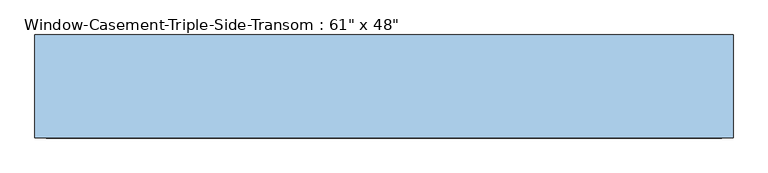
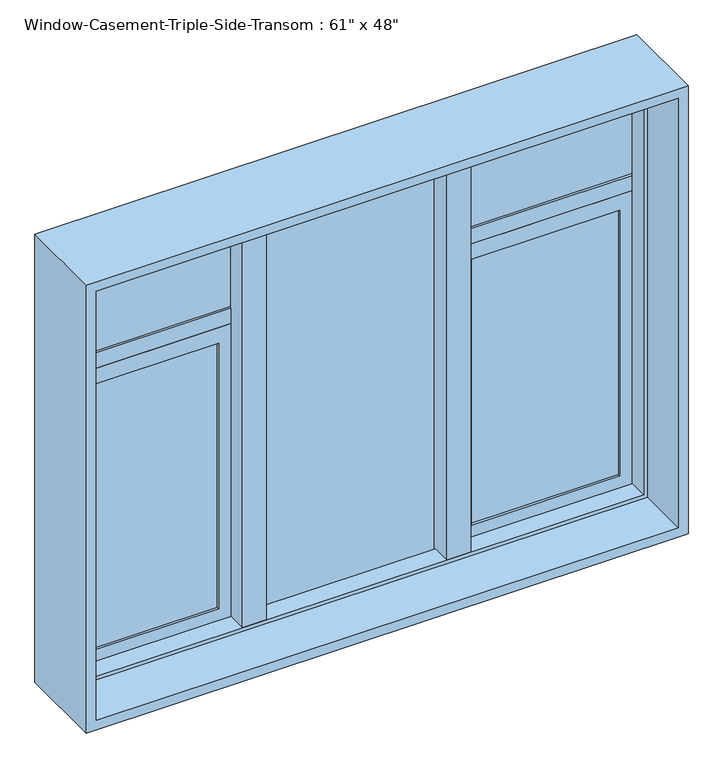
"""IFC4 building model written with IfcOpenShell, lengths in millimetres: window geometry."""

from ifc_helpers import new_model, si_unit, frame, origin, place, context, project, spatial, polyline, outline, extrude, faceted_brep, source, transform, mapped, element, save


def window_1a7cbd99(model_context):
    return source(origin(), model_context, "Body", "SolidModel", [
        faceted_brep([(-749.3, 73.025, 2108.2), (-749.3, 114.3, 2108.2), (749.3, 114.3, 2108.2), (749.3, 73.025, 2108.2), (-739.1796875, 22.225, 2098.0796875), (-739.1796875, 73.025, 2098.0796875), (739.1796875, 73.025, 2098.0796875), (739.1796875, 22.225, 2098.0796875), (-749.3, -114.3, 2108.2), (-749.3, 22.225, 2108.2), (749.3, 22.225, 2108.2), (749.3, -114.3, 2108.2), (-774.7, 114.3, 2133.6), (-774.7, -114.3, 2133.6), (774.7, -114.3, 2133.6), (774.7, 114.3, 2133.6), (749.3, 114.3, 939.8), (749.3, 73.025, 939.8), (739.1796875, 73.025, 949.9203125), (739.1796875, 22.225, 949.9203125), (749.3, 22.225, 939.8), (749.3, -114.3, 939.8), (774.7, -114.3, 914.4), (774.7, 114.3, 914.4), (-749.3, 114.3, 939.8), (-749.3, 73.025, 939.8), (-739.1796875, 73.025, 949.9203125), (-739.1796875, 22.225, 949.9203125), (-749.3, 22.225, 939.8), (-749.3, -114.3, 939.8), (-774.7, -114.3, 914.4), (-774.7, 114.3, 914.4)], [[[0, 1, 2, 3]], [[4, 5, 6, 7]], [[8, 9, 10, 11]], [[12, 13, 14, 15]], [[3, 2, 16, 17]], [[7, 6, 18, 19]], [[11, 10, 20, 21]], [[15, 14, 22, 23]], [[17, 16, 24, 25]], [[19, 18, 26, 27]], [[21, 20, 28, 29]], [[23, 22, 30, 31]], [[25, 24, 1, 0]], [[3, 17, 25, 0], [5, 26, 18, 6]], [[27, 26, 5, 4]], [[9, 28, 20, 10], [7, 19, 27, 4]], [[29, 28, 9, 8]], [[13, 30, 22, 14], [11, 21, 29, 8]], [[31, 30, 13, 12]], [[15, 23, 31, 12], [1, 24, 16, 2]]]),
        extrude(outline(polyline([(-232.8333333, 111.125), (-232.8333333, 22.225), (-293.7536458, 22.225), (-293.7536458, 73.025), (-283.6333333, 73.025), (-283.6333333, 111.125), (-232.8333333, 111.125)])), frame((0.0, 0.0, 939.8), z_axis=(0.0, 0.0, 1.0), x_axis=(1.0, 0.0, 0.0)), (0.0, 0.0, 1.0), 1168.4),
        extrude(outline(polyline([(283.6333333, 111.125), (283.6333333, 73.025), (293.7536458, 73.025), (293.7536458, 22.225), (232.8333333, 22.225), (232.8333333, 111.125), (283.6333333, 111.125)])), frame((0.0, 0.0, 939.8), z_axis=(0.0, 0.0, 1.0), x_axis=(1.0, 0.0, 0.0)), (0.0, 0.0, 1.0), 1168.4),
        extrude(outline(polyline([(1746.9048438, 283.6333333), (939.8, 283.6333333), (939.8, 749.3), (1746.9048438, 749.3), (1746.9048438, 283.6333333)]), holes=[polyline([(1705.0345313, 707.4296875), (981.6703125, 707.4296875), (981.6703125, 325.5036458), (1705.0345313, 325.5036458), (1705.0345313, 707.4296875)])]), frame((0.0, 73.025, 0.0), z_axis=(0.0, 1.0, 0.0), x_axis=(0.0, 0.0, 1.0)), (0.0, 0.0, 1.0), 31.75),
        extrude(outline(polyline([(1746.9048438, -749.3), (939.8, -749.3), (939.8, -283.6333333), (1746.9048438, -283.6333333), (1746.9048438, -749.3)]), holes=[polyline([(1705.0345313, -325.5036458), (981.6703125, -325.5036458), (981.6703125, -707.4296875), (1705.0345313, -707.4296875), (1705.0345313, -325.5036458)])]), frame((0.0, 73.025, 0.0), z_axis=(0.0, 1.0, 0.0), x_axis=(0.0, 0.0, 1.0)), (0.0, 0.0, 1.0), 31.75),
        extrude(outline(polyline([(-325.5036458, 98.425), (-325.5036458, 92.075), (-707.4296875, 92.075), (-707.4296875, 98.425), (-325.5036458, 98.425)])), frame((0.0, 0.0, 981.6703125), z_axis=(0.0, 0.0, 1.0), x_axis=(1.0, 0.0, 0.0)), (0.0, 0.0, 1.0), 723.3642188),
        extrude(outline(polyline([(-325.5036458, 85.725), (-325.5036458, 79.375), (-707.4296875, 79.375), (-707.4296875, 85.725), (-325.5036458, 85.725)])), frame((0.0, 0.0, 981.6703125), z_axis=(0.0, 0.0, 1.0), x_axis=(1.0, 0.0, 0.0)), (0.0, 0.0, 1.0), 723.3642188),
        extrude(outline(polyline([(707.4296875, 98.425), (707.4296875, 92.075), (325.5036458, 92.075), (325.5036458, 98.425), (707.4296875, 98.425)])), frame((0.0, 0.0, 981.6703125), z_axis=(0.0, 0.0, 1.0), x_axis=(1.0, 0.0, 0.0)), (0.0, 0.0, 1.0), 723.3642188),
        extrude(outline(polyline([(707.4296875, 85.725), (707.4296875, 79.375), (325.5036458, 79.375), (325.5036458, 85.725), (707.4296875, 85.725)])), frame((0.0, 0.0, 981.6703125), z_axis=(0.0, 0.0, 1.0), x_axis=(1.0, 0.0, 0.0)), (0.0, 0.0, 1.0), 723.3642188),
        extrude(outline(polyline([(749.3, 104.775), (749.3, 73.025), (283.6333333, 73.025), (283.6333333, 104.775), (749.3, 104.775)])), frame((0.0, 0.0, 1746.9048438), z_axis=(0.0, 0.0, 1.0), x_axis=(1.0, 0.0, 0.0)), (0.0, 0.0, 1.0), 41.8703125),
        extrude(outline(polyline([(232.8333333, 98.425), (232.8333333, 92.075), (-232.8333333, 92.075), (-232.8333333, 98.425), (232.8333333, 98.425)])), frame((0.0, 0.0, 939.8), z_axis=(0.0, 0.0, 1.0), x_axis=(1.0, 0.0, 0.0)), (0.0, 0.0, 1.0), 1168.4),
        extrude(outline(polyline([(232.8333333, 85.725), (232.8333333, 79.375), (-232.8333333, 79.375), (-232.8333333, 85.725), (232.8333333, 85.725)])), frame((0.0, 0.0, 939.8), z_axis=(0.0, 0.0, 1.0), x_axis=(1.0, 0.0, 0.0)), (0.0, 0.0, 1.0), 1168.4),
        extrude(outline(polyline([(-283.6333333, 104.775), (-283.6333333, 73.025), (-749.3, 73.025), (-749.3, 104.775), (-283.6333333, 104.775)])), frame((0.0, 0.0, 1746.9048438), z_axis=(0.0, 0.0, 1.0), x_axis=(1.0, 0.0, 0.0)), (0.0, 0.0, 1.0), 41.8703125),
        extrude(outline(polyline([(-283.6333333, 98.425), (-283.6333333, 92.075), (-749.3, 92.075), (-749.3, 98.425), (-283.6333333, 98.425)])), frame((0.0, 0.0, 1788.7751562), z_axis=(0.0, 0.0, 1.0), x_axis=(1.0, 0.0, 0.0)), (0.0, 0.0, 1.0), 319.4248438),
        extrude(outline(polyline([(-283.6333333, 85.725), (-283.6333333, 79.375), (-749.3, 79.375), (-749.3, 85.725), (-283.6333333, 85.725)])), frame((0.0, 0.0, 1788.7751562), z_axis=(0.0, 0.0, 1.0), x_axis=(1.0, 0.0, 0.0)), (0.0, 0.0, 1.0), 319.4248438),
        extrude(outline(polyline([(749.3, 98.425), (749.3, 92.075), (283.6333333, 92.075), (283.6333333, 98.425), (749.3, 98.425)])), frame((0.0, 0.0, 1788.7751562), z_axis=(0.0, 0.0, 1.0), x_axis=(1.0, 0.0, 0.0)), (0.0, 0.0, 1.0), 319.4248438),
        extrude(outline(polyline([(749.3, 85.725), (749.3, 79.375), (283.6333333, 79.375), (283.6333333, 85.725), (749.3, 85.725)])), frame((0.0, 0.0, 1788.7751562), z_axis=(0.0, 0.0, 1.0), x_axis=(1.0, 0.0, 0.0)), (0.0, 0.0, 1.0), 319.4248438),
    ])


if __name__ == "__main__":
    model = new_model("IFC4")
    model_context = context("Model", 3, world=origin())
    ifc_project = project(units=[si_unit("LENGTHUNIT", "METRE", prefix="MILLI")], contexts=[model_context])
    site = spatial("IfcSite", under=ifc_project)
    building = spatial("IfcBuilding", under=site)
    placement = place(None, origin())
    window_shape = window_1a7cbd99(model_context)
    element("IfcWindow", 1, ObjectType="Window-Casement-Triple-Side-Transom : 61\" x 48\"", at=placement, inside=building, context=model_context, shape_type="MappedRepresentation", body=[
        mapped(window_shape, transform((0.0, 0.0, 0.0), x_axis=(1.0, 0.0, 0.0), y_axis=(0.0, 1.0, 0.0), z_axis=(0.0, 0.0, 1.0))),
    ])
    save(model, "model.ifc")

# Revit data of these elements
# Type "Window-Casement-Triple-Side-Transom : 61\" x 48\""
#   Type Mark = "23"
#   Fire Rating = "0.5h"
#   Assembly Code = "B2020100"
#   Analytic Construction = "Double glazing - domestic"
#   Window Width = 1' - 8.33333"
#   Window Inset [instance default] = 0' - 0 5/8"
#   Wall Thickness [instance default] = 0' - 6"
#   Visual Light Transmittance = 0.81
#   Transom Height Ratio = 0.3
#   Thermal Resistance (R) = 1.8146 (h·ft²·°F)/BTU
#   Solar Heat Gain Coefficient = 0.76
#   Rough Width = 5' - 1 1/2"
#   Rough Height = 4' - 0 1/2"
#   Open Window Height = 2' - 9.6"
#   Heat Transfer Coefficient (U) = 0.5511 BTU/(h·ft²·°F)
#   Height = 4' - 0"
#   Transom Height = 1' - 2.4"
#   Frame Gap 3 [instance default] = 0' - 1 83/128"
#   Frame Gap 2 [instance default] = 0' - 0 5/8"
#   Frame Gap 1 = 0' - 1 51/128"
#   Default Sill Height = 3' - 0"
#   Width = 5' - 1"
#   Frame Material = Metal - Aluminum
#   Glass Panel Material = Glass
#   Wall Closure = (empty or 0)
# Element 1 (IfcWindow, "Window-Casement-Triple-Side-Transom : 61\" x 48\"")
#   Wall Thickness = 0' - 9"
#   Materials on its faces: "Metal - Aluminum", "Glass"
# Materials
#   "Metal - Aluminum": class "Metal", colour RGB 247 247 247, transparency 0
#   "Glass": class "Glass", colour RGB 154 182 205, transparency 0.85, Description = "Soda Lime Glass", Cost = 0
